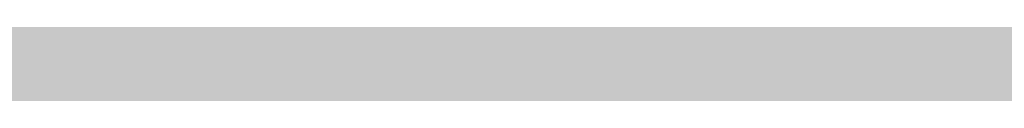
# Model space of a CAD drawing. Units: millimetres. Extents: x 0 to 2267, y 0 to 1823.
# Tile 204 of 256: x 1841.442 to 1842.748, y 1127.306 to 1127.384. Entities that reach past the tile are written whole.
import ezdxf

# ---------------------------------------------------------------- set-up
doc = ezdxf.new("R2010")
doc.units = ezdxf.units.MM
doc.header["$MEASUREMENT"] = 0
doc.layers.add('M-DIMS', color=2, linetype='Continuous', lineweight=25)
doc.layers.add('M-HATC', color=252, linetype='Continuous', lineweight=18)
doc.styles.get("Standard").update_dxf_attribs({"font": 'arial.ttf'})
doc.dimstyles.get("Standard").update_dxf_attribs({"dimtxt": 7, "dimasz": 4, "dimexe": 0.18, "dimexo": 0.0625, "dimgap": 0.09, "dimtad": 0, "dimdec": 0, "dimzin": 0, "dimdsep": 46, "dimtxsty": 'Standard', "dimcen": 0.09, "dimadec": 0, "dimazin": 0, "dimtfac": 1, "dimtdec": 0, "dimtofl": 0, "dimtmove": 0, "dimatfit": 3, "dimfxl": 1, "dimtolj": 1, "dimtzin": 0, "dimarcsym": 0})

# ---------------------------------------------------------------- blocks, each defined once
blk = doc.blocks.new('*D1')
at = {"layer": 'Defpoints', "color": 0, "transparency": 16777216}
for p in [(1593.4289, 1127.4171), (1843.4289, 1127.4171), (1843.4289, 955.6278)]:
    blk.add_point(p, dxfattribs=at)
at = {"layer": 'M-DIMS', "color": 0, "lineweight": -2, "transparency": 16777216}
for p, q in [((1593.4289, 1127.3546), (1593.4289, 955.4478)), ((1843.4289, 1127.3546), (1843.4289, 955.4478)), ((1597.4289, 955.6278), (1710.5582, 955.6278)), ((1839.4289, 955.6278), (1726.2996, 955.6278))]:
    blk.add_line(p, q, dxfattribs=at)
at = {"layer": 'M-DIMS', "color": 0, "transparency": 16777216}
for points in [[(1597.4289, 956.2944), (1597.4289, 954.9611), (1593.4289, 955.6278)], [(1839.4289, 956.2944), (1839.4289, 954.9611), (1843.4289, 955.6278)]]:
    blk.add_solid(points, dxfattribs=at)
at = {"layer": 'M-DIMS', "color": 0, "transparency": 16777216, "insert": (1718.4289, 955.6278), "char_height": 7, "attachment_point": 5}
blk.add_mtext('\\A1;250', dxfattribs=at)

msp = doc.modelspace()

# ---------------------------------------------------------------- hatches: boundary and pattern name
at = {"layer": 'M-HATC'}
h = msp.add_hatch(color=256, dxfattribs=at)
h.dxf.hatch_style = 1
h.paths.add_polyline_path([(2055.771, 1603.062), (1381.0868, 1603.062), (1381.0868, 1598.062), (2055.771, 1598.062)])
h.paths.add_polyline_path([(2055.771, 1598.062), (1381.0868, 1598.062), (1381.0868, 1593.062), (2055.771, 1593.062)])
h.paths.add_polyline_path([(2051.3074, 1536.7609), (1385.5504, 1536.7609), (1385.5504, 1526.7609), (1387.5504, 1526.7609), (1388.5366, 1525.0528), (1385.3319, 1521.2335), (1385.3319, 1521.2226), (2050.2542, 1522.7491), (2048.3212, 1525.0528), (2049.3074, 1526.7609), (2051.3074, 1526.7609)])
edge = h.paths.add_edge_path()
edge.add_arc((1847.5345, 1379.1492), 135, 222.603061, 222.890851, ccw=False)
edge.add_line((1748.1663, 1287.7656), (1683.0921, 1287.7656))
edge.add_arc((1583.7239, 1379.1492), 135, 317.109149, 317.396939, ccw=False)
edge.add_arc((1678.9686, 1290.6707), 5, 222.8909, 317.1091, ccw=False)
edge.add_arc((1774.2133, 1379.1492), 135, 222.603061, 222.890851, ccw=False)
edge.add_line((1674.8451, 1287.7656), (1609.7709, 1287.7656))
edge.add_arc((1510.4027, 1379.1492), 135, 317.109149, 317.396939, ccw=False)
edge.add_arc((1605.6474, 1290.6707), 5, 222.8909, 317.1091, ccw=False)
edge.add_arc((1700.8921, 1379.1492), 135, 222.603061, 222.890851, ccw=False)
edge.add_line((1601.5239, 1287.7656), (1536.4497, 1287.7656))
edge.add_arc((1437.0815, 1379.1492), 135, 317.109149, 317.396939, ccw=False)
edge.add_arc((1532.3262, 1290.6707), 5, 222.8909, 317.1091, ccw=False)
edge.add_arc((1627.5709, 1379.1492), 135, 222.603061, 222.890851, ccw=False)
edge.add_line((1528.2027, 1287.7656), (1505.9289, 1287.7656))
edge.add_spline(control_points=[(1505.9289, 1287.7656), (1504.2622, 1287.7656), (1504.2622, 1282.7656), (1505.9289, 1282.7656)], knot_values=[0, 0, 0, 0, 5, 5, 5, 5], degree=3, periodic=0)
edge.add_line((1505.9289, 1282.7656), (1930.9289, 1282.7656))
edge.add_spline(control_points=[(1930.9289, 1282.7656), (1932.5956, 1282.7656), (1932.5956, 1287.7656), (1930.9289, 1287.7656)], knot_values=[0, 0, 0, 0, 5, 5, 5, 5], degree=3, periodic=0)
edge.add_line((1930.9289, 1287.7656), (1903.0557, 1287.7656))
edge.add_arc((1803.6875, 1379.1492), 135, 317.109149, 317.396939, ccw=False)
edge.add_arc((1898.9322, 1290.6707), 5, 222.8909, 317.1091, ccw=False)
edge.add_arc((1994.1769, 1379.1492), 135, 222.603061, 222.890851, ccw=False)
edge.add_line((1894.8087, 1287.7656), (1829.7345, 1287.7656))
edge.add_arc((1730.3663, 1379.1492), 135, 317.109149, 317.396939, ccw=False)
edge.add_arc((1825.611, 1290.6707), 5, 222.8909, 317.1091, ccw=False)
edge.add_arc((1920.8557, 1379.1492), 135, 222.603061, 222.890851, ccw=False)
edge.add_line((1821.4875, 1287.7656), (1756.4133, 1287.7656))
edge.add_arc((1657.0451, 1379.1492), 135, 317.109149, 317.396939, ccw=False)
edge.add_arc((1752.2898, 1290.6707), 5, 222.8909, 317.1091, ccw=False)
edge = h.paths.add_edge_path()
edge.add_spline(control_points=[(1843.4289, 1227.2475), (1845.0956, 1227.2475), (1845.0956, 1232.2475), (1843.4289, 1232.2475)], knot_values=[0, 0, 0, 0, 5, 5, 5, 5], degree=3, periodic=0)
edge.add_line((1843.4289, 1232.2475), (1593.4289, 1232.2475))
edge.add_spline(control_points=[(1593.4289, 1232.2475), (1591.7622, 1232.2475), (1591.7622, 1227.2475), (1593.4289, 1227.2475)], knot_values=[0, 0, 0, 0, 5, 5, 5, 5], degree=3, periodic=0)
edge.add_line((1593.4289, 1227.2475), (1843.4289, 1227.2475))
h.paths.add_polyline_path([(1905.9289, 1127.4171), (1530.9289, 1127.4171, 0.414214), (1520.9289, 1117.4171), (1530.9289, 1117.4171), (1915.9289, 1117.4171, 0.414214)])
edge = h.paths.add_edge_path()
edge.add_arc((1397.0858, 1498.4078), 12.7299, 90.78215, 190.87871, ccw=False)
edge.add_line((1396.912, 1511.1365), (1428.0097, 1511.3488))
edge.add_line((1428.0097, 1511.3488), (1433.0097, 1511.3488))
edge.add_line((1433.0097, 1511.3488), (1434.439, 1511.3488))
edge.add_arc((1419.474, 1498.0804), 20, 41.561, 74.08211)
edge.add_line((1424.9592, 1517.3135), (1399.9351, 1517.2561))
edge.add_spline(control_points=[(1399.9307, 1517.2561), (1399.884, 1517.2131), (1399.8328, 1517.1689), (1399.7774, 1517.1236)], knot_values=[11.567499, 11.567499, 11.567499, 11.567499, 11.814249, 11.814249, 11.814249, 11.814249], degree=3, periodic=0)
edge.add_spline(control_points=[(1399.6328, 1517.0099), (1399.5831, 1516.9721), (1399.5307, 1516.9338), (1399.4759, 1516.8947)], knot_values=[11.167718, 11.167718, 11.167718, 11.167718, 11.365188, 11.365188, 11.365188, 11.365188], degree=3, periodic=0)
edge.add_spline(control_points=[(1399.3398, 1516.8001), (1399.1514, 1516.6719), (1398.9384, 1516.5377), (1398.704, 1516.3994)], knot_values=[10.376405, 10.376405, 10.376405, 10.376405, 11.00994, 11.00994, 11.00994, 11.00994], degree=3, periodic=0)
edge.add_spline(control_points=[(1398.6572, 1516.3719), (1398.5789, 1516.326), (1398.4983, 1516.2797), (1398.4155, 1516.2331)], knot_values=[10.125175, 10.125175, 10.125175, 10.125175, 10.334406, 10.334406, 10.334406, 10.334406], degree=3, periodic=0)
edge.add_spline(control_points=[(1398.2642, 1516.1487), (1398.196, 1516.1111), (1398.1263, 1516.0732), (1398.0555, 1516.0351)], knot_values=[9.832246, 9.832246, 9.832246, 9.832246, 9.999658, 9.999658, 9.999658, 9.999658], degree=3, periodic=0)
edge.add_spline(control_points=[(1397.9987, 1516.0048), (1397.7312, 1515.8621), (1397.446, 1515.7171), (1397.1466, 1515.5714)], knot_values=[9.161808, 9.161808, 9.161808, 9.161808, 9.787769, 9.787769, 9.787769, 9.787769], degree=3, periodic=0)
edge.add_spline(control_points=[(1397.1466, 1515.5714), (1396.8418, 1515.423), (1396.5222, 1515.274), (1396.1914, 1515.1262)], knot_values=[8.524455, 8.524455, 8.524455, 8.524455, 9.161808, 9.161808, 9.161808, 9.161808], degree=3, periodic=0)
edge.add_spline(control_points=[(1396.0777, 1515.0756), (1395.9854, 1515.0348), (1395.8922, 1514.994), (1395.7983, 1514.9534)], knot_values=[8.275193, 8.275193, 8.275193, 8.275193, 8.451726, 8.451726, 8.451726, 8.451726], degree=3, periodic=0)
edge.add_spline(control_points=[(1395.6018, 1514.8691), (1395.4997, 1514.8257), (1395.3968, 1514.7824), (1395.2932, 1514.7394)], knot_values=[7.962917, 7.962917, 7.962917, 7.962917, 8.152764, 8.152764, 8.152764, 8.152764], degree=3, periodic=0)
edge.add_spline(control_points=[(1395.2116, 1514.7057), (1394.8278, 1514.5475), (1394.4345, 1514.3929), (1394.0364, 1514.2442)], knot_values=[7.21254, 7.21254, 7.21254, 7.21254, 7.913148, 7.913148, 7.913148, 7.913148], degree=3, periodic=0)
edge.add_spline(control_points=[(1394.0364, 1514.2442), (1393.7076, 1514.1214), (1393.3754, 1514.0027), (1393.0427, 1513.8895)], knot_values=[6.633733, 6.633733, 6.633733, 6.633733, 7.21254, 7.21254, 7.21254, 7.21254], degree=3, periodic=0)
edge.add_spline(control_points=[(1392.8214, 1513.815), (1392.7198, 1513.7812), (1392.6181, 1513.7479), (1392.5166, 1513.7152)], knot_values=[6.328796, 6.328796, 6.328796, 6.328796, 6.505493, 6.505493, 6.505493, 6.505493], degree=3, periodic=0)
edge.add_spline(control_points=[(1392.5166, 1513.7152), (1392.3187, 1513.6515), (1392.1212, 1513.59), (1391.9244, 1513.531)], knot_values=[5.984605, 5.984605, 5.984605, 5.984605, 6.328796, 6.328796, 6.328796, 6.328796], degree=3, periodic=0)
edge.add_spline(control_points=[(1391.7915, 1513.4915), (1391.3122, 1513.3501), (1390.8384, 1513.2239), (1390.3784, 1513.1171)], knot_values=[5.066697, 5.066697, 5.066697, 5.066697, 5.907055, 5.907055, 5.907055, 5.907055], degree=3, periodic=0)
edge.add_spline(control_points=[(1390.3784, 1513.1171), (1390.1797, 1513.071), (1389.9836, 1513.0284), (1389.7907, 1512.9899)], knot_values=[4.70367, 4.70367, 4.70367, 4.70367, 5.066695, 5.066695, 5.066695, 5.066695], degree=3, periodic=0)
edge.add_spline(control_points=[(1389.422, 1512.9204), (1389.2459, 1512.8892), (1389.0729, 1512.8617), (1388.9036, 1512.8381)], knot_values=[4.130571, 4.130571, 4.130571, 4.130571, 4.469816, 4.469816, 4.469816, 4.469816], degree=3, periodic=0)
edge.add_spline(control_points=[(1388.9036, 1512.8381), (1388.591, 1512.7946), (1388.2911, 1512.7644), (1388.0071, 1512.7494)], knot_values=[3.504031, 3.504031, 3.504031, 3.504031, 4.130571, 4.130571, 4.130571, 4.130571], degree=3, periodic=0)
edge.add_spline(control_points=[(1387.9356, 1512.7459), (1387.8538, 1512.7423), (1387.7733, 1512.74), (1387.6944, 1512.739)], knot_values=[3.268866, 3.268866, 3.268866, 3.268866, 3.451164, 3.451164, 3.451164, 3.451164], degree=3, periodic=0)
edge.add_spline(control_points=[(1387.3351, 1512.7443), (1387.2076, 1512.7499), (1387.0847, 1512.7597), (1386.967, 1512.7739)], knot_values=[2.670686, 2.670686, 2.670686, 2.670686, 2.984, 2.984, 2.984, 2.984], degree=3, periodic=0)
edge.add_spline(control_points=[(1386.8327, 1512.7922), (1386.8209, 1512.7941), (1386.8092, 1512.7959), (1386.7975, 1512.7979)], knot_values=[2.516981, 2.516981, 2.516981, 2.516981, 2.549528, 2.549528, 2.549528, 2.549528], degree=3, periodic=0)
edge.add_spline(control_points=[(1386.4526, 1512.8735), (1386.4257, 1512.881), (1386.3993, 1512.889), (1386.3733, 1512.8972)], knot_values=[2.095869, 2.095869, 2.095869, 2.095869, 2.17941, 2.17941, 2.17941, 2.17941], degree=3, periodic=0)
edge.add_spline(control_points=[(1386.0691, 1513.0189), (1386.0634, 1513.0217), (1386.0577, 1513.0246), (1386.052, 1513.0275)], knot_values=[1.72453, 1.72453, 1.72453, 1.72453, 1.745933, 1.745933, 1.745933, 1.745933], degree=3, periodic=0)
edge.add_arc((1399.474, 1498.0804), 20, 131.82432, 180)
edge.add_arc((1630.3336, 1505.5484), 250.9708, 181.705176, 236.427975)
edge.add_arc((1605.3399, 1483.3044), 218.7822, 238.660829, 243.34961)
edge.add_arc((1647.0911, 1510.3592), 262.8986, 183.129836, 237.853442, ccw=False)
h.paths.add_polyline_path([(1406.5369, 1391.9644, 0.149382), (1491.5506, 1296.4418, -0.129517)], flags=17)
edge = h.paths.add_edge_path()
edge.add_arc((2037.3838, 1498.0804), 20, 0, 48.26587)
edge.add_spline(control_points=[(2050.6973, 1513.0052), (2050.6512, 1512.9847), (2050.6034, 1512.9655), (2050.5539, 1512.9477)], knot_values=[1.835652, 1.835652, 1.835652, 1.835652, 2.000781, 2.000781, 2.000781, 2.000781], degree=3, periodic=0)
edge.add_spline(control_points=[(2050.4616, 1512.9166), (2050.479, 1512.9221), (2050.4963, 1512.9277), (2050.5133, 1512.9335)], knot_values=[2.045477, 2.045477, 2.045477, 2.045477, 2.101389, 2.101389, 2.101389, 2.101389], degree=3, periodic=0)
edge.add_spline(control_points=[(2050.129, 1512.8342), (2050.1984, 1512.8473), (2050.2657, 1512.8623), (2050.3308, 1512.8792)], knot_values=[2.237629, 2.237629, 2.237629, 2.237629, 2.435841, 2.435841, 2.435841, 2.435841], degree=3, periodic=0)
edge.add_spline(control_points=[(2050.0946, 1512.8278), (2050.1061, 1512.8299), (2050.1176, 1512.832), (2050.129, 1512.8342)], knot_values=[2.435841, 2.435841, 2.435841, 2.435841, 2.468321, 2.468321, 2.468321, 2.468321], degree=3, periodic=0)
edge.add_spline(control_points=[(2049.7843, 1512.7851), (2049.8552, 1512.7922), (2049.9243, 1512.8008), (2049.9917, 1512.8109)], knot_values=[2.563852, 2.563852, 2.563852, 2.563852, 2.748541, 2.748541, 2.748541, 2.748541], degree=3, periodic=0)
edge.add_spline(control_points=[(2049.4052, 1512.7617), (2049.5364, 1512.7653), (2049.6629, 1512.773), (2049.7843, 1512.7851)], knot_values=[2.748541, 2.748541, 2.748541, 2.748541, 3.064882, 3.064882, 3.064882, 3.064882], degree=3, periodic=0)
edge.add_spline(control_points=[(2049.1698, 1512.7597), (2049.2336, 1512.7591), (2049.2965, 1512.7594), (2049.3584, 1512.7606)], knot_values=[3.102309, 3.102309, 3.102309, 3.102309, 3.2503, 3.2503, 3.2503, 3.2503], degree=3, periodic=0)
edge.add_spline(control_points=[(2048.8573, 1512.7691), (2048.9638, 1512.7638), (2049.068, 1512.7606), (2049.1698, 1512.7597)], knot_values=[3.2503, 3.2503, 3.2503, 3.2503, 3.486069, 3.486069, 3.486069, 3.486069], degree=3, periodic=0)
edge.add_spline(control_points=[(2048.6924, 1512.7789), (2048.3729, 1512.8009), (2048.0345, 1512.8411), (2047.6817, 1512.897)], knot_values=[3.606429, 3.606429, 3.606429, 3.606429, 4.2989, 4.2989, 4.2989, 4.2989], degree=3, periodic=0)
edge.add_spline(control_points=[(2047.6817, 1512.897), (2047.5458, 1512.9185), (2047.4077, 1512.9424), (2047.2678, 1512.9685)], knot_values=[4.2989, 4.2989, 4.2989, 4.2989, 4.565769, 4.565769, 4.565769, 4.565769], degree=3, periodic=0)
edge.add_spline(control_points=[(2047.2678, 1512.9685), (2047.1449, 1512.9914), (2047.0207, 1513.016), (2046.8951, 1513.0422)], knot_values=[4.565769, 4.565769, 4.565769, 4.565769, 4.799971, 4.799971, 4.799971, 4.799971], degree=3, periodic=0)
edge.add_spline(control_points=[(2046.8951, 1513.0422), (2046.5286, 1513.1188), (2046.1513, 1513.209), (2045.7676, 1513.3107)], knot_values=[4.799971, 4.799971, 4.799971, 4.799971, 5.483718, 5.483718, 5.483718, 5.483718], degree=3, periodic=0)
edge.add_spline(control_points=[(2045.7676, 1513.3107), (2045.3724, 1513.4154), (2044.9704, 1513.5322), (2044.5662, 1513.6588)], knot_values=[5.483718, 5.483718, 5.483718, 5.483718, 6.187866, 6.187866, 6.187866, 6.187866], degree=3, periodic=0)
edge.add_spline(control_points=[(2044.5662, 1513.6588), (2044.4149, 1513.7061), (2044.2633, 1513.7549), (2044.1116, 1513.8048)], knot_values=[6.187866, 6.187866, 6.187866, 6.187866, 6.451551, 6.451551, 6.451551, 6.451551], degree=3, periodic=0)
edge.add_spline(control_points=[(2044.1116, 1513.8048), (2043.9967, 1513.8427), (2043.8817, 1513.8813), (2043.7668, 1513.9205)], knot_values=[6.451551, 6.451551, 6.451551, 6.451551, 6.651434, 6.651434, 6.651434, 6.651434], degree=3, periodic=0)
edge.add_spline(control_points=[(2043.7668, 1513.9205), (2043.3716, 1514.0554), (2042.9774, 1514.1979), (2042.5886, 1514.3458)], knot_values=[6.651434, 6.651434, 6.651434, 6.651434, 7.338879, 7.338879, 7.338879, 7.338879], degree=3, periodic=0)
edge.add_spline(control_points=[(2042.5886, 1514.3458), (2042.1643, 1514.5071), (2041.7465, 1514.6749), (2041.3409, 1514.846)], knot_values=[7.338879, 7.338879, 7.338879, 7.338879, 8.089209, 8.089209, 8.089209, 8.089209], degree=3, periodic=0)
edge.add_spline(control_points=[(2041.3409, 1514.846), (2041.1028, 1514.9465), (2040.869, 1515.0481), (2040.6405, 1515.1502)], knot_values=[8.089209, 8.089209, 8.089209, 8.089209, 8.529587, 8.529587, 8.529587, 8.529587], degree=3, periodic=0)
edge.add_spline(control_points=[(2040.51, 1515.2089), (2040.0824, 1515.4022), (2039.6747, 1515.5971), (2039.295, 1515.7894)], knot_values=[8.613818, 8.613818, 8.613818, 8.613818, 9.44571, 9.44571, 9.44571, 9.44571], degree=3, periodic=0)
edge.add_spline(control_points=[(2039.295, 1515.7894), (2039.0618, 1515.9075), (2038.8391, 1516.0246), (2038.6288, 1516.1398)], knot_values=[9.44571, 9.44571, 9.44571, 9.44571, 9.956404, 9.956404, 9.956404, 9.956404], degree=3, periodic=0)
edge.add_spline(control_points=[(2038.6288, 1516.1398), (2038.5187, 1516.2001), (2038.4121, 1516.2598), (2038.309, 1516.3189)], knot_values=[9.956404, 9.956404, 9.956404, 9.956404, 10.223542, 10.223542, 10.223542, 10.223542], degree=3, periodic=0)
edge.add_spline(control_points=[(2038.309, 1516.3189), (2038.2138, 1516.3735), (2038.1216, 1516.4276), (2038.0328, 1516.481)], knot_values=[10.223542, 10.223542, 10.223542, 10.223542, 10.47051, 10.47051, 10.47051, 10.47051], degree=3, periodic=0)
edge.add_spline(control_points=[(2038.0328, 1516.481), (2037.7855, 1516.6296), (2037.5639, 1516.773), (2037.3722, 1516.909)], knot_values=[10.47051, 10.47051, 10.47051, 10.47051, 11.15767, 11.15767, 11.15767, 11.15767], degree=3, periodic=0)
edge.add_spline(control_points=[(2037.3722, 1516.909), (2037.2789, 1516.9752), (2037.1927, 1517.0396), (2037.1142, 1517.102)], knot_values=[11.15767, 11.15767, 11.15767, 11.15767, 11.49227, 11.49227, 11.49227, 11.49227], degree=3, periodic=0)
edge.add_spline(control_points=[(2036.8564, 1517.3259), (2036.9148, 1517.2692), (2036.9814, 1517.2103), (2037.0557, 1517.1492)], knot_values=[11.577341, 11.577341, 11.577341, 11.577341, 11.91035, 11.91035, 11.91035, 11.91035], degree=3, periodic=0)
edge.add_spline(control_points=[(2036.8074, 1517.3748), (2036.823, 1517.3587), (2036.8393, 1517.3424), (2036.8564, 1517.3259)], knot_values=[11.91035, 11.91035, 11.91035, 11.91035, 12.007402, 12.007402, 12.007402, 12.007402], degree=3, periodic=0)
edge.add_spline(control_points=[(2036.7017, 1517.494), (2036.7104, 1517.483), (2036.7196, 1517.4719), (2036.7291, 1517.4606)], knot_values=[12.184155, 12.184155, 12.184155, 12.184155, 12.255409, 12.255409, 12.255409, 12.255409], degree=3, periodic=0)
edge.add_spline(control_points=[(2036.6159, 1517.6205), (2036.62, 1517.613), (2036.6243, 1517.6055), (2036.6289, 1517.5979)], knot_values=[12.487913, 12.487913, 12.487913, 12.487913, 12.541035, 12.541035, 12.541035, 12.541035], degree=3, periodic=0)
edge.add_spline(control_points=[(2036.5635, 1517.786), (2036.5637, 1517.7794), (2036.5642, 1517.7726), (2036.565, 1517.7658)], knot_values=[12.911761, 12.911761, 12.911761, 12.911761, 12.968286, 12.968286, 12.968286, 12.968286], degree=3, periodic=0)
edge.add_spline(control_points=[(2036.6166, 1517.9304), (2036.6125, 1517.9259), (2036.6086, 1517.9212), (2036.6049, 1517.9165)], knot_values=[13.382527, 13.382527, 13.382527, 13.382527, 13.433791, 13.433791, 13.433791, 13.433791], degree=3, periodic=0)
edge.add_spline(control_points=[(2036.749, 1518.017), (2036.7361, 1518.0116), (2036.7239, 1518.006), (2036.7124, 1518.0002)], knot_values=[13.726299, 13.726299, 13.726299, 13.726299, 13.809928, 13.809928, 13.809928, 13.809928], degree=3, periodic=0)
edge.add_spline(control_points=[(2036.8604, 1518.0528), (2036.8386, 1518.0474), (2036.8181, 1518.0416), (2036.7988, 1518.0353)], knot_values=[13.910887, 13.910887, 13.910887, 13.910887, 14.02153, 14.02153, 14.02153, 14.02153], degree=3, periodic=0)
edge.add_line((2036.9639, 1518.0804), (2032.3838, 1518.0804))
edge.add_line((2032.3838, 1518.0804), (2027.3838, 1518.0804))
edge.add_line((2027.3838, 1518.0804), (2022.3838, 1518.0804))
edge.add_line((2022.3838, 1518.0804), (2017.3838, 1518.0804))
edge.add_arc((2017.3838, 1498.0804), 20, 90, 138.439)
edge.add_line((2002.4188, 1511.3488), (2003.8481, 1511.3488))
edge.add_line((2003.8481, 1511.3488), (2008.8481, 1511.3488))
edge.add_line((2008.8481, 1511.3488), (2039.772, 1511.1377))
edge.add_arc((2039.772, 1498.4078), 12.7299, -10.87871, 90, ccw=False)
edge.add_arc((1789.7668, 1510.3592), 262.8986, 302.146558, 356.870164, ccw=False)
edge.add_arc((1831.5179, 1483.3044), 218.7822, 296.65039, 301.339171)
edge.add_arc((1806.5242, 1505.5484), 250.9708, 303.572025, 358.294824)
h.paths.add_polyline_path([(2030.321, 1391.9644, -0.129517), (1945.3072, 1296.4418, 0.149382)], flags=17)
edge = h.paths.add_edge_path()
edge.add_spline(control_points=[(2037.2464, 1518.0821), (2037.2898, 1518.081), (2037.3355, 1518.0804), (2037.3838, 1518.0804)], knot_values=[0.000012, 0.000012, 0.000012, 0.000012, 0.144754, 0.144754, 0.144754, 0.144754], degree=3, periodic=0)
edge.add_line((2037.3357, 1518.0804), (2037.0096, 1518.0804))
edge.add_spline(control_points=[(2037.0096, 1518.0804), (2036.9822, 1518.0768), (2036.956, 1518.0727), (2036.9312, 1518.0681)], knot_values=[14.13465, 14.13465, 14.13465, 14.13465, 14.247197, 14.247197, 14.247197, 14.247197], degree=3, periodic=0)
edge.add_spline(control_points=[(2036.9312, 1518.0681), (2036.9276, 1518.0674), (2036.9241, 1518.0667), (2036.9205, 1518.0661)], knot_values=[14.118315, 14.118315, 14.118315, 14.118315, 14.13465, 14.13465, 14.13465, 14.13465], degree=3, periodic=0)
edge.add_spline(control_points=[(2036.9205, 1518.0661), (2036.9118, 1518.0644), (2036.9032, 1518.0626), (2036.8948, 1518.0608)], knot_values=[14.078086, 14.078086, 14.078086, 14.078086, 14.118315, 14.118315, 14.118315, 14.118315], degree=3, periodic=0)
edge.add_spline(control_points=[(2036.8948, 1518.0608), (2036.883, 1518.0583), (2036.8716, 1518.0556), (2036.8604, 1518.0528)], knot_values=[14.02153, 14.02153, 14.02153, 14.02153, 14.078086, 14.078086, 14.078086, 14.078086], degree=3, periodic=0)
edge.add_spline(control_points=[(2036.8604, 1518.0528), (2036.8386, 1518.0474), (2036.8181, 1518.0416), (2036.7988, 1518.0353)], knot_values=[13.910887, 13.910887, 13.910887, 13.910887, 14.02153, 14.02153, 14.02153, 14.02153], degree=3, periodic=0)
edge.add_spline(control_points=[(2036.7988, 1518.0353), (2036.7981, 1518.035), (2036.7974, 1518.0348), (2036.7967, 1518.0346)], knot_values=[13.906906, 13.906906, 13.906906, 13.906906, 13.910887, 13.910887, 13.910887, 13.910887], degree=3, periodic=0)
edge.add_spline(control_points=[(2036.7967, 1518.0346), (2036.7882, 1518.0318), (2036.7799, 1518.0289), (2036.7719, 1518.0259)], knot_values=[13.857826, 13.857826, 13.857826, 13.857826, 13.906906, 13.906906, 13.906906, 13.906906], degree=3, periodic=0)
edge.add_spline(control_points=[(2036.7719, 1518.0259), (2036.764, 1518.023), (2036.7564, 1518.02), (2036.749, 1518.017)], knot_values=[13.809928, 13.809928, 13.809928, 13.809928, 13.857826, 13.857826, 13.857826, 13.857826], degree=3, periodic=0)
edge.add_spline(control_points=[(2036.749, 1518.017), (2036.7361, 1518.0116), (2036.7239, 1518.006), (2036.7124, 1518.0002)], knot_values=[13.726299, 13.726299, 13.726299, 13.726299, 13.809928, 13.809928, 13.809928, 13.809928], degree=3, periodic=0)
edge.add_spline(control_points=[(2036.7124, 1518.0002), (2036.7121, 1518), (2036.7118, 1517.9999), (2036.7115, 1517.9997)], knot_values=[13.723993, 13.723993, 13.723993, 13.723993, 13.726299, 13.726299, 13.726299, 13.726299], degree=3, periodic=0)
edge.add_spline(control_points=[(2036.7115, 1517.9997), (2036.7063, 1517.9971), (2036.7013, 1517.9944), (2036.6965, 1517.9917)], knot_values=[13.686536, 13.686536, 13.686536, 13.686536, 13.723993, 13.723993, 13.723993, 13.723993], degree=3, periodic=0)
edge.add_spline(control_points=[(2036.6965, 1517.9917), (2036.6919, 1517.9891), (2036.6874, 1517.9865), (2036.6831, 1517.9839)], knot_values=[13.651251, 13.651251, 13.651251, 13.651251, 13.686536, 13.686536, 13.686536, 13.686536], degree=3, periodic=0)
edge.add_spline(control_points=[(2036.6831, 1517.9839), (2036.6764, 1517.9798), (2036.67, 1517.9757), (2036.6639, 1517.9714)], knot_values=[13.596804, 13.596804, 13.596804, 13.596804, 13.651251, 13.651251, 13.651251, 13.651251], degree=3, periodic=0)
edge.add_spline(control_points=[(2036.6639, 1517.9714), (2036.6636, 1517.9712), (2036.6633, 1517.9709), (2036.6629, 1517.9707)], knot_values=[13.593956, 13.593956, 13.593956, 13.593956, 13.596804, 13.596804, 13.596804, 13.596804], degree=3, periodic=0)
edge.add_spline(control_points=[(2036.6629, 1517.9707), (2036.6603, 1517.9689), (2036.6577, 1517.967), (2036.6552, 1517.9651)], knot_values=[13.570322, 13.570322, 13.570322, 13.570322, 13.593956, 13.593956, 13.593956, 13.593956], degree=3, periodic=0)
edge.add_spline(control_points=[(2036.6552, 1517.9651), (2036.6525, 1517.9631), (2036.6499, 1517.9611), (2036.6474, 1517.9591)], knot_values=[13.545477, 13.545477, 13.545477, 13.545477, 13.570322, 13.570322, 13.570322, 13.570322], degree=3, periodic=0)
edge.add_spline(control_points=[(2036.6474, 1517.9591), (2036.6472, 1517.9589), (2036.6471, 1517.9588), (2036.6469, 1517.9587)], knot_values=[13.543931, 13.543931, 13.543931, 13.543931, 13.545477, 13.545477, 13.545477, 13.545477], degree=3, periodic=0)
edge.add_spline(control_points=[(2036.6469, 1517.9587), (2036.6412, 1517.9541), (2036.6358, 1517.9494), (2036.6307, 1517.9447)], knot_values=[13.488237, 13.488237, 13.488237, 13.488237, 13.543931, 13.543931, 13.543931, 13.543931], degree=3, periodic=0)
edge.add_spline(control_points=[(2036.6307, 1517.9447), (2036.6282, 1517.9423), (2036.6257, 1517.9399), (2036.6233, 1517.9374)], knot_values=[13.460307, 13.460307, 13.460307, 13.460307, 13.488237, 13.488237, 13.488237, 13.488237], degree=3, periodic=0)
edge.add_spline(control_points=[(2036.6233, 1517.9374), (2036.6215, 1517.9356), (2036.6198, 1517.9338), (2036.6181, 1517.932)], knot_values=[13.439712, 13.439712, 13.439712, 13.439712, 13.460307, 13.460307, 13.460307, 13.460307], degree=3, periodic=0)
edge.add_spline(control_points=[(2036.6181, 1517.932), (2036.6176, 1517.9315), (2036.6171, 1517.9309), (2036.6166, 1517.9304)], knot_values=[13.433791, 13.433791, 13.433791, 13.433791, 13.439712, 13.439712, 13.439712, 13.439712], degree=3, periodic=0)
edge.add_spline(control_points=[(2036.6166, 1517.9304), (2036.6125, 1517.9259), (2036.6086, 1517.9212), (2036.6049, 1517.9165)], knot_values=[13.382527, 13.382527, 13.382527, 13.382527, 13.433791, 13.433791, 13.433791, 13.433791], degree=3, periodic=0)
edge.add_spline(control_points=[(2036.6049, 1517.9165), (2036.6026, 1517.9135), (2036.6004, 1517.9104), (2036.5982, 1517.9074)], knot_values=[13.350017, 13.350017, 13.350017, 13.350017, 13.382527, 13.382527, 13.382527, 13.382527], degree=3, periodic=0)
edge.add_spline(control_points=[(2036.5982, 1517.9074), (2036.5972, 1517.9059), (2036.5962, 1517.9043), (2036.5952, 1517.9028)], knot_values=[13.333922, 13.333922, 13.333922, 13.333922, 13.350017, 13.350017, 13.350017, 13.350017], degree=3, periodic=0)
edge.add_spline(control_points=[(2036.5952, 1517.9028), (2036.5945, 1517.9018), (2036.5939, 1517.9009), (2036.5933, 1517.8999)], knot_values=[13.323828, 13.323828, 13.323828, 13.323828, 13.333922, 13.333922, 13.333922, 13.333922], degree=3, periodic=0)
edge.add_spline(control_points=[(2036.5933, 1517.8999), (2036.5905, 1517.8955), (2036.5879, 1517.8909), (2036.5855, 1517.8864)], knot_values=[13.277545, 13.277545, 13.277545, 13.277545, 13.323828, 13.323828, 13.323828, 13.323828], degree=3, periodic=0)
edge.add_spline(control_points=[(2036.5855, 1517.8864), (2036.5836, 1517.8827), (2036.5817, 1517.8789), (2036.5801, 1517.8751)], knot_values=[13.240119, 13.240119, 13.240119, 13.240119, 13.277545, 13.277545, 13.277545, 13.277545], degree=3, periodic=0)
edge.add_spline(control_points=[(2036.5801, 1517.8751), (2036.5795, 1517.8739), (2036.579, 1517.8727), (2036.5785, 1517.8715)], knot_values=[13.228211, 13.228211, 13.228211, 13.228211, 13.240119, 13.240119, 13.240119, 13.240119], degree=3, periodic=0)
edge.add_spline(control_points=[(2036.5785, 1517.8715), (2036.578, 1517.8702), (2036.5774, 1517.869), (2036.5769, 1517.8677)], knot_values=[13.215717, 13.215717, 13.215717, 13.215717, 13.228211, 13.228211, 13.228211, 13.228211], degree=3, periodic=0)
edge.add_spline(control_points=[(2036.5769, 1517.8677), (2036.5755, 1517.864), (2036.5741, 1517.8603), (2036.5729, 1517.8565)], knot_values=[13.179847, 13.179847, 13.179847, 13.179847, 13.215717, 13.215717, 13.215717, 13.215717], degree=3, periodic=0)
edge.add_spline(control_points=[(2036.5729, 1517.8565), (2036.5713, 1517.8515), (2036.5699, 1517.8464), (2036.5687, 1517.8413)], knot_values=[13.132017, 13.132017, 13.132017, 13.132017, 13.179847, 13.179847, 13.179847, 13.179847], degree=3, periodic=0)
edge.add_spline(control_points=[(2036.5687, 1517.8413), (2036.5684, 1517.8402), (2036.5682, 1517.8392), (2036.568, 1517.8382)], knot_values=[13.122482, 13.122482, 13.122482, 13.122482, 13.132017, 13.132017, 13.132017, 13.132017], degree=3, periodic=0)
edge.add_spline(control_points=[(2036.568, 1517.8382), (2036.5676, 1517.8363), (2036.5672, 1517.8345), (2036.5669, 1517.8327)], knot_values=[13.105592, 13.105592, 13.105592, 13.105592, 13.122482, 13.122482, 13.122482, 13.122482], degree=3, periodic=0)
edge.add_spline(control_points=[(2036.5669, 1517.8327), (2036.5662, 1517.8292), (2036.5657, 1517.8257), (2036.5652, 1517.8222)], knot_values=[13.074063, 13.074063, 13.074063, 13.074063, 13.105592, 13.105592, 13.105592, 13.105592], degree=3, periodic=0)
edge.add_spline(control_points=[(2036.5652, 1517.8222), (2036.5652, 1517.8222), (2036.5652, 1517.8222), (2036.5652, 1517.8222)], knot_values=[13.074043, 13.074043, 13.074043, 13.074043, 13.074063, 13.074063, 13.074063, 13.074063], degree=3, periodic=0)
edge.add_spline(control_points=[(2036.5652, 1517.8222), (2036.5644, 1517.8164), (2036.5639, 1517.8106), (2036.5636, 1517.8046)], knot_values=[13.021884, 13.021884, 13.021884, 13.021884, 13.074043, 13.074043, 13.074043, 13.074043], degree=3, periodic=0)
edge.add_spline(control_points=[(2036.5636, 1517.8046), (2036.5636, 1517.804), (2036.5636, 1517.8034), (2036.5635, 1517.8028)], knot_values=[13.01674, 13.01674, 13.01674, 13.01674, 13.021884, 13.021884, 13.021884, 13.021884], degree=3, periodic=0)
edge.add_spline(control_points=[(2036.5635, 1517.8028), (2036.5634, 1517.8005), (2036.5634, 1517.7982), (2036.5634, 1517.7958)], knot_values=[12.996438, 12.996438, 12.996438, 12.996438, 13.01674, 13.01674, 13.01674, 13.01674], degree=3, periodic=0)
edge.add_spline(control_points=[(2036.5634, 1517.7958), (2036.5633, 1517.7926), (2036.5634, 1517.7893), (2036.5635, 1517.786)], knot_values=[12.968286, 12.968286, 12.968286, 12.968286, 12.996438, 12.996438, 12.996438, 12.996438], degree=3, periodic=0)
edge.add_spline(control_points=[(2036.5635, 1517.786), (2036.5637, 1517.7794), (2036.5642, 1517.7726), (2036.565, 1517.7658)], knot_values=[12.911761, 12.911761, 12.911761, 12.911761, 12.968286, 12.968286, 12.968286, 12.968286], degree=3, periodic=0)
edge.add_spline(control_points=[(2036.565, 1517.7658), (2036.565, 1517.7657), (2036.565, 1517.7656), (2036.565, 1517.7656)], knot_values=[12.911017, 12.911017, 12.911017, 12.911017, 12.911761, 12.911761, 12.911761, 12.911761], degree=3, periodic=0)
edge.add_spline(control_points=[(2036.565, 1517.7656), (2036.5654, 1517.7625), (2036.5658, 1517.7593), (2036.5663, 1517.7562)], knot_values=[12.88528, 12.88528, 12.88528, 12.88528, 12.911017, 12.911017, 12.911017, 12.911017], degree=3, periodic=0)
edge.add_spline(control_points=[(2036.5663, 1517.7562), (2036.5667, 1517.7534), (2036.5672, 1517.7506), (2036.5677, 1517.7478)], knot_values=[12.862519, 12.862519, 12.862519, 12.862519, 12.88528, 12.88528, 12.88528, 12.88528], degree=3, periodic=0)
edge.add_spline(control_points=[(2036.5677, 1517.7478), (2036.5678, 1517.7474), (2036.5679, 1517.7469), (2036.568, 1517.7465)], knot_values=[12.858885, 12.858885, 12.858885, 12.858885, 12.862519, 12.862519, 12.862519, 12.862519], degree=3, periodic=0)
edge.add_spline(control_points=[(2036.568, 1517.7465), (2036.5692, 1517.7399), (2036.5707, 1517.7332), (2036.5724, 1517.7264)], knot_values=[12.8053, 12.8053, 12.8053, 12.8053, 12.858885, 12.858885, 12.858885, 12.858885], degree=3, periodic=0)
edge.add_spline(control_points=[(2036.5724, 1517.7264), (2036.5734, 1517.7226), (2036.5745, 1517.7187), (2036.5756, 1517.7149)], knot_values=[12.775176, 12.775176, 12.775176, 12.775176, 12.8053, 12.8053, 12.8053, 12.8053], degree=3, periodic=0)
edge.add_spline(control_points=[(2036.5756, 1517.7149), (2036.5763, 1517.7125), (2036.577, 1517.7102), (2036.5778, 1517.7078)], knot_values=[12.756759, 12.756759, 12.756759, 12.756759, 12.775176, 12.775176, 12.775176, 12.775176], degree=3, periodic=0)
edge.add_spline(control_points=[(2036.5778, 1517.7078), (2036.5781, 1517.7067), (2036.5784, 1517.7057), (2036.5787, 1517.7047)], knot_values=[12.748742, 12.748742, 12.748742, 12.748742, 12.756759, 12.756759, 12.756759, 12.756759], degree=3, periodic=0)
edge.add_spline(control_points=[(2036.5787, 1517.7047), (2036.5808, 1517.6983), (2036.5831, 1517.6919), (2036.5856, 1517.6854)], knot_values=[12.69959, 12.69959, 12.69959, 12.69959, 12.748742, 12.748742, 12.748742, 12.748742], degree=3, periodic=0)
edge.add_spline(control_points=[(2036.5856, 1517.6854), (2036.5876, 1517.68), (2036.5898, 1517.6746), (2036.5921, 1517.6692)], knot_values=[12.659038, 12.659038, 12.659038, 12.659038, 12.69959, 12.69959, 12.69959, 12.69959], degree=3, periodic=0)
edge.add_spline(control_points=[(2036.5921, 1517.6692), (2036.594, 1517.6648), (2036.5959, 1517.6605), (2036.5979, 1517.6561)], knot_values=[12.626806, 12.626806, 12.626806, 12.626806, 12.659038, 12.659038, 12.659038, 12.659038], degree=3, periodic=0)
edge.add_spline(control_points=[(2036.5979, 1517.6561), (2036.5984, 1517.6551), (2036.5989, 1517.6541), (2036.5993, 1517.6531)], knot_values=[12.619394, 12.619394, 12.619394, 12.619394, 12.626806, 12.626806, 12.626806, 12.626806], degree=3, periodic=0)
edge.add_spline(control_points=[(2036.5993, 1517.6531), (2036.6043, 1517.6424), (2036.6099, 1517.6315), (2036.6159, 1517.6205)], knot_values=[12.541039, 12.541039, 12.541039, 12.541039, 12.619394, 12.619394, 12.619394, 12.619394], degree=3, periodic=0)
edge.add_spline(control_points=[(2036.6159, 1517.6205), (2036.6159, 1517.6205), (2036.6159, 1517.6205), (2036.6159, 1517.6205)], knot_values=[12.541035, 12.541035, 12.541035, 12.541035, 12.541039, 12.541039, 12.541039, 12.541039], degree=3, periodic=0)
edge.add_spline(control_points=[(2036.6159, 1517.6205), (2036.62, 1517.613), (2036.6243, 1517.6055), (2036.6289, 1517.5979)], knot_values=[12.487913, 12.487913, 12.487913, 12.487913, 12.541035, 12.541035, 12.541035, 12.541035], degree=3, periodic=0)
edge.add_spline(control_points=[(2036.6289, 1517.5979), (2036.6326, 1517.5916), (2036.6365, 1517.5853), (2036.6406, 1517.5789)], knot_values=[12.443982, 12.443982, 12.443982, 12.443982, 12.487913, 12.487913, 12.487913, 12.487913], degree=3, periodic=0)
edge.add_spline(control_points=[(2036.6406, 1517.5789), (2036.6414, 1517.5776), (2036.6423, 1517.5763), (2036.6431, 1517.5749)], knot_values=[12.434996, 12.434996, 12.434996, 12.434996, 12.443982, 12.443982, 12.443982, 12.443982], degree=3, periodic=0)
edge.add_spline(control_points=[(2036.6431, 1517.5749), (2036.6531, 1517.5596), (2036.6639, 1517.5439), (2036.6756, 1517.528)], knot_values=[12.329647, 12.329647, 12.329647, 12.329647, 12.434996, 12.434996, 12.434996, 12.434996], degree=3, periodic=0)
edge.add_spline(control_points=[(2036.6756, 1517.528), (2036.6839, 1517.5168), (2036.6925, 1517.5055), (2036.7017, 1517.494)], knot_values=[12.255409, 12.255409, 12.255409, 12.255409, 12.329647, 12.329647, 12.329647, 12.329647], degree=3, periodic=0)
edge.add_spline(control_points=[(2036.7017, 1517.494), (2036.7104, 1517.483), (2036.7196, 1517.4719), (2036.7291, 1517.4606)], knot_values=[12.184155, 12.184155, 12.184155, 12.184155, 12.255409, 12.255409, 12.255409, 12.255409], degree=3, periodic=0)
edge.add_spline(control_points=[(2036.7291, 1517.4606), (2036.7436, 1517.4435), (2036.759, 1517.4262), (2036.7753, 1517.4085)], knot_values=[12.075961, 12.075961, 12.075961, 12.075961, 12.184155, 12.184155, 12.184155, 12.184155], degree=3, periodic=0)
edge.add_spline(control_points=[(2036.7753, 1517.4085), (2036.7763, 1517.4075), (2036.7773, 1517.4064), (2036.7783, 1517.4054)], knot_values=[12.069502, 12.069502, 12.069502, 12.069502, 12.075961, 12.075961, 12.075961, 12.075961], degree=3, periodic=0)
edge.add_spline(control_points=[(2036.7783, 1517.4054), (2036.7877, 1517.3953), (2036.7974, 1517.385), (2036.8074, 1517.3748)], knot_values=[12.007402, 12.007402, 12.007402, 12.007402, 12.069502, 12.069502, 12.069502, 12.069502], degree=3, periodic=0)
edge.add_spline(control_points=[(2036.8074, 1517.3748), (2036.823, 1517.3587), (2036.8393, 1517.3424), (2036.8564, 1517.3259)], knot_values=[11.91035, 11.91035, 11.91035, 11.91035, 12.007402, 12.007402, 12.007402, 12.007402], degree=3, periodic=0)
edge.add_spline(control_points=[(2036.8564, 1517.3259), (2036.9148, 1517.2692), (2036.9814, 1517.2103), (2037.0557, 1517.1492)], knot_values=[11.577341, 11.577341, 11.577341, 11.577341, 11.91035, 11.91035, 11.91035, 11.91035], degree=3, periodic=0)
edge.add_spline(control_points=[(2037.0557, 1517.1492), (2037.0747, 1517.1336), (2037.0942, 1517.1179), (2037.1142, 1517.102)], knot_values=[11.49227, 11.49227, 11.49227, 11.49227, 11.577341, 11.577341, 11.577341, 11.577341], degree=3, periodic=0)
edge.add_spline(control_points=[(2037.1142, 1517.102), (2037.1927, 1517.0396), (2037.2789, 1516.9752), (2037.3722, 1516.909)], knot_values=[11.15767, 11.15767, 11.15767, 11.15767, 11.49227, 11.49227, 11.49227, 11.49227], degree=3, periodic=0)
edge.add_spline(control_points=[(2037.3722, 1516.909), (2037.5639, 1516.773), (2037.7855, 1516.6296), (2038.0328, 1516.481)], knot_values=[10.47051, 10.47051, 10.47051, 10.47051, 11.15767, 11.15767, 11.15767, 11.15767], degree=3, periodic=0)
edge.add_spline(control_points=[(2038.0328, 1516.481), (2038.1216, 1516.4276), (2038.2138, 1516.3735), (2038.309, 1516.3189)], knot_values=[10.223542, 10.223542, 10.223542, 10.223542, 10.47051, 10.47051, 10.47051, 10.47051], degree=3, periodic=0)
edge.add_spline(control_points=[(2038.309, 1516.3189), (2038.4121, 1516.2598), (2038.5187, 1516.2001), (2038.6288, 1516.1398)], knot_values=[9.956404, 9.956404, 9.956404, 9.956404, 10.223542, 10.223542, 10.223542, 10.223542], degree=3, periodic=0)
edge.add_spline(control_points=[(2038.6288, 1516.1398), (2038.8391, 1516.0246), (2039.0618, 1515.9075), (2039.295, 1515.7894)], knot_values=[9.44571, 9.44571, 9.44571, 9.44571, 9.956404, 9.956404, 9.956404, 9.956404], degree=3, periodic=0)
edge.add_spline(control_points=[(2039.295, 1515.7894), (2039.6747, 1515.5971), (2040.0824, 1515.4022), (2040.51, 1515.2089)], knot_values=[8.613818, 8.613818, 8.613818, 8.613818, 9.44571, 9.44571, 9.44571, 9.44571], degree=3, periodic=0)
edge.add_spline(control_points=[(2040.51, 1515.2089), (2040.5533, 1515.1893), (2040.5968, 1515.1697), (2040.6405, 1515.1502)], knot_values=[8.529587, 8.529587, 8.529587, 8.529587, 8.613818, 8.613818, 8.613818, 8.613818], degree=3, periodic=0)
edge.add_spline(control_points=[(2040.6405, 1515.1502), (2040.869, 1515.0481), (2041.1028, 1514.9465), (2041.3409, 1514.846)], knot_values=[8.089209, 8.089209, 8.089209, 8.089209, 8.529587, 8.529587, 8.529587, 8.529587], degree=3, periodic=0)
edge.add_spline(control_points=[(2041.3409, 1514.846), (2041.7465, 1514.6749), (2042.1643, 1514.5071), (2042.5886, 1514.3458)], knot_values=[7.338879, 7.338879, 7.338879, 7.338879, 8.089209, 8.089209, 8.089209, 8.089209], degree=3, periodic=0)
edge.add_spline(control_points=[(2042.5886, 1514.3458), (2042.9774, 1514.1979), (2043.3716, 1514.0554), (2043.7668, 1513.9205)], knot_values=[6.651434, 6.651434, 6.651434, 6.651434, 7.338879, 7.338879, 7.338879, 7.338879], degree=3, periodic=0)
edge.add_spline(control_points=[(2043.7668, 1513.9205), (2043.8817, 1513.8813), (2043.9967, 1513.8427), (2044.1116, 1513.8048)], knot_values=[6.451551, 6.451551, 6.451551, 6.451551, 6.651434, 6.651434, 6.651434, 6.651434], degree=3, periodic=0)
edge.add_spline(control_points=[(2044.1116, 1513.8048), (2044.2633, 1513.7549), (2044.4149, 1513.7061), (2044.5662, 1513.6588)], knot_values=[6.187866, 6.187866, 6.187866, 6.187866, 6.451551, 6.451551, 6.451551, 6.451551], degree=3, periodic=0)
edge.add_spline(control_points=[(2044.5662, 1513.6588), (2044.9704, 1513.5322), (2045.3724, 1513.4154), (2045.7676, 1513.3107)], knot_values=[5.483718, 5.483718, 5.483718, 5.483718, 6.187866, 6.187866, 6.187866, 6.187866], degree=3, periodic=0)
edge.add_spline(control_points=[(2045.7676, 1513.3107), (2046.1513, 1513.209), (2046.5286, 1513.1188), (2046.8951, 1513.0422)], knot_values=[4.799971, 4.799971, 4.799971, 4.799971, 5.483718, 5.483718, 5.483718, 5.483718], degree=3, periodic=0)
edge.add_spline(control_points=[(2046.8951, 1513.0422), (2047.0207, 1513.016), (2047.1449, 1512.9914), (2047.2678, 1512.9685)], knot_values=[4.565769, 4.565769, 4.565769, 4.565769, 4.799971, 4.799971, 4.799971, 4.799971], degree=3, periodic=0)
edge.add_spline(control_points=[(2047.2678, 1512.9685), (2047.4077, 1512.9424), (2047.5458, 1512.9185), (2047.6817, 1512.897)], knot_values=[4.2989, 4.2989, 4.2989, 4.2989, 4.565769, 4.565769, 4.565769, 4.565769], degree=3, periodic=0)
edge.add_spline(control_points=[(2047.6817, 1512.897), (2048.0345, 1512.8411), (2048.3729, 1512.8009), (2048.6924, 1512.7789)], knot_values=[3.606429, 3.606429, 3.606429, 3.606429, 4.2989, 4.2989, 4.2989, 4.2989], degree=3, periodic=0)
edge.add_spline(control_points=[(2048.6924, 1512.7789), (2048.7479, 1512.7751), (2048.8029, 1512.7718), (2048.8573, 1512.7691)], knot_values=[3.486069, 3.486069, 3.486069, 3.486069, 3.606429, 3.606429, 3.606429, 3.606429], degree=3, periodic=0)
edge.add_spline(control_points=[(2048.8573, 1512.7691), (2048.9638, 1512.7638), (2049.068, 1512.7606), (2049.1698, 1512.7597)], knot_values=[3.2503, 3.2503, 3.2503, 3.2503, 3.486069, 3.486069, 3.486069, 3.486069], degree=3, periodic=0)
edge.add_spline(control_points=[(2049.1698, 1512.7597), (2049.2336, 1512.7591), (2049.2965, 1512.7594), (2049.3584, 1512.7606)], knot_values=[3.102309, 3.102309, 3.102309, 3.102309, 3.2503, 3.2503, 3.2503, 3.2503], degree=3, periodic=0)
edge.add_spline(control_points=[(2049.3584, 1512.7606), (2049.3741, 1512.7609), (2049.3897, 1512.7613), (2049.4052, 1512.7617)], knot_values=[3.064882, 3.064882, 3.064882, 3.064882, 3.102309, 3.102309, 3.102309, 3.102309], degree=3, periodic=0)
edge.add_spline(control_points=[(2049.4052, 1512.7617), (2049.5364, 1512.7653), (2049.6629, 1512.773), (2049.7843, 1512.7851)], knot_values=[2.748541, 2.748541, 2.748541, 2.748541, 3.064882, 3.064882, 3.064882, 3.064882], degree=3, periodic=0)
edge.add_spline(control_points=[(2049.7843, 1512.7851), (2049.8552, 1512.7922), (2049.9243, 1512.8008), (2049.9917, 1512.8109)], knot_values=[2.563852, 2.563852, 2.563852, 2.563852, 2.748541, 2.748541, 2.748541, 2.748541], degree=3, periodic=0)
edge.add_spline(control_points=[(2049.9917, 1512.8109), (2050.0265, 1512.8161), (2050.0608, 1512.8218), (2050.0946, 1512.8278)], knot_values=[2.468321, 2.468321, 2.468321, 2.468321, 2.563852, 2.563852, 2.563852, 2.563852], degree=3, periodic=0)
edge.add_spline(control_points=[(2050.0946, 1512.8278), (2050.1061, 1512.8299), (2050.1176, 1512.832), (2050.129, 1512.8342)], knot_values=[2.435841, 2.435841, 2.435841, 2.435841, 2.468321, 2.468321, 2.468321, 2.468321], degree=3, periodic=0)
edge.add_spline(control_points=[(2050.129, 1512.8342), (2050.1984, 1512.8473), (2050.2657, 1512.8623), (2050.3308, 1512.8792)], knot_values=[2.237629, 2.237629, 2.237629, 2.237629, 2.435841, 2.435841, 2.435841, 2.435841], degree=3, periodic=0)
edge.add_spline(control_points=[(2050.3308, 1512.8792), (2050.3754, 1512.8908), (2050.4191, 1512.9032), (2050.4616, 1512.9166)], knot_values=[2.101389, 2.101389, 2.101389, 2.101389, 2.237629, 2.237629, 2.237629, 2.237629], degree=3, periodic=0)
edge.add_spline(control_points=[(2050.4616, 1512.9166), (2050.479, 1512.9221), (2050.4963, 1512.9277), (2050.5133, 1512.9335)], knot_values=[2.045477, 2.045477, 2.045477, 2.045477, 2.101389, 2.101389, 2.101389, 2.101389], degree=3, periodic=0)
edge.add_spline(control_points=[(2050.5133, 1512.9335), (2050.527, 1512.9382), (2050.5405, 1512.9429), (2050.5539, 1512.9477)], knot_values=[2.000781, 2.000781, 2.000781, 2.000781, 2.045477, 2.045477, 2.045477, 2.045477], degree=3, periodic=0)
edge.add_spline(control_points=[(2050.5539, 1512.9477), (2050.6034, 1512.9655), (2050.6512, 1512.9847), (2050.6973, 1513.0052)], knot_values=[1.835652, 1.835652, 1.835652, 1.835652, 2.000781, 2.000781, 2.000781, 2.000781], degree=3, periodic=0)
edge.add_arc((2037.3838, 1498.0804), 20, 48.26587, 90.12993)
edge = h.paths.add_edge_path(flags=16)
edge.add_spline(control_points=[(1386.1389, 1512.9859), (1388.92, 1511.7395), (1398.0387, 1515.5187), (1399.9307, 1517.2561)], knot_values=[1.831046, 1.831046, 1.831046, 1.831046, 11.814249, 11.814249, 11.814249, 11.814249], degree=3, periodic=0)
edge.add_line((1399.9307, 1517.2561), (1393.7435, 1517.2419))
edge.add_arc((1399.474, 1498.0804), 20, 106.6501, 131.8173)

# ---------------------------------------------------------------- dimensions: what is measured, and where the dimension line sits
at = {"layer": 'M-DIMS'}
dim = msp.add_linear_dim(base=(1843.4289, 955.6278), p1=(1593.4289, 1127.4171), p2=(1843.4289, 1127.4171), dimstyle='Standard', override={"dimclrd": 0, "dimclre": 0, "dimclrt": 0}, dxfattribs=at)
dim.commit()
dim.dimension.update_dxf_attribs({"geometry": '*D1', "text_midpoint": (1718.4289, 955.6278)})

doc.saveas('drawing.dxf')
